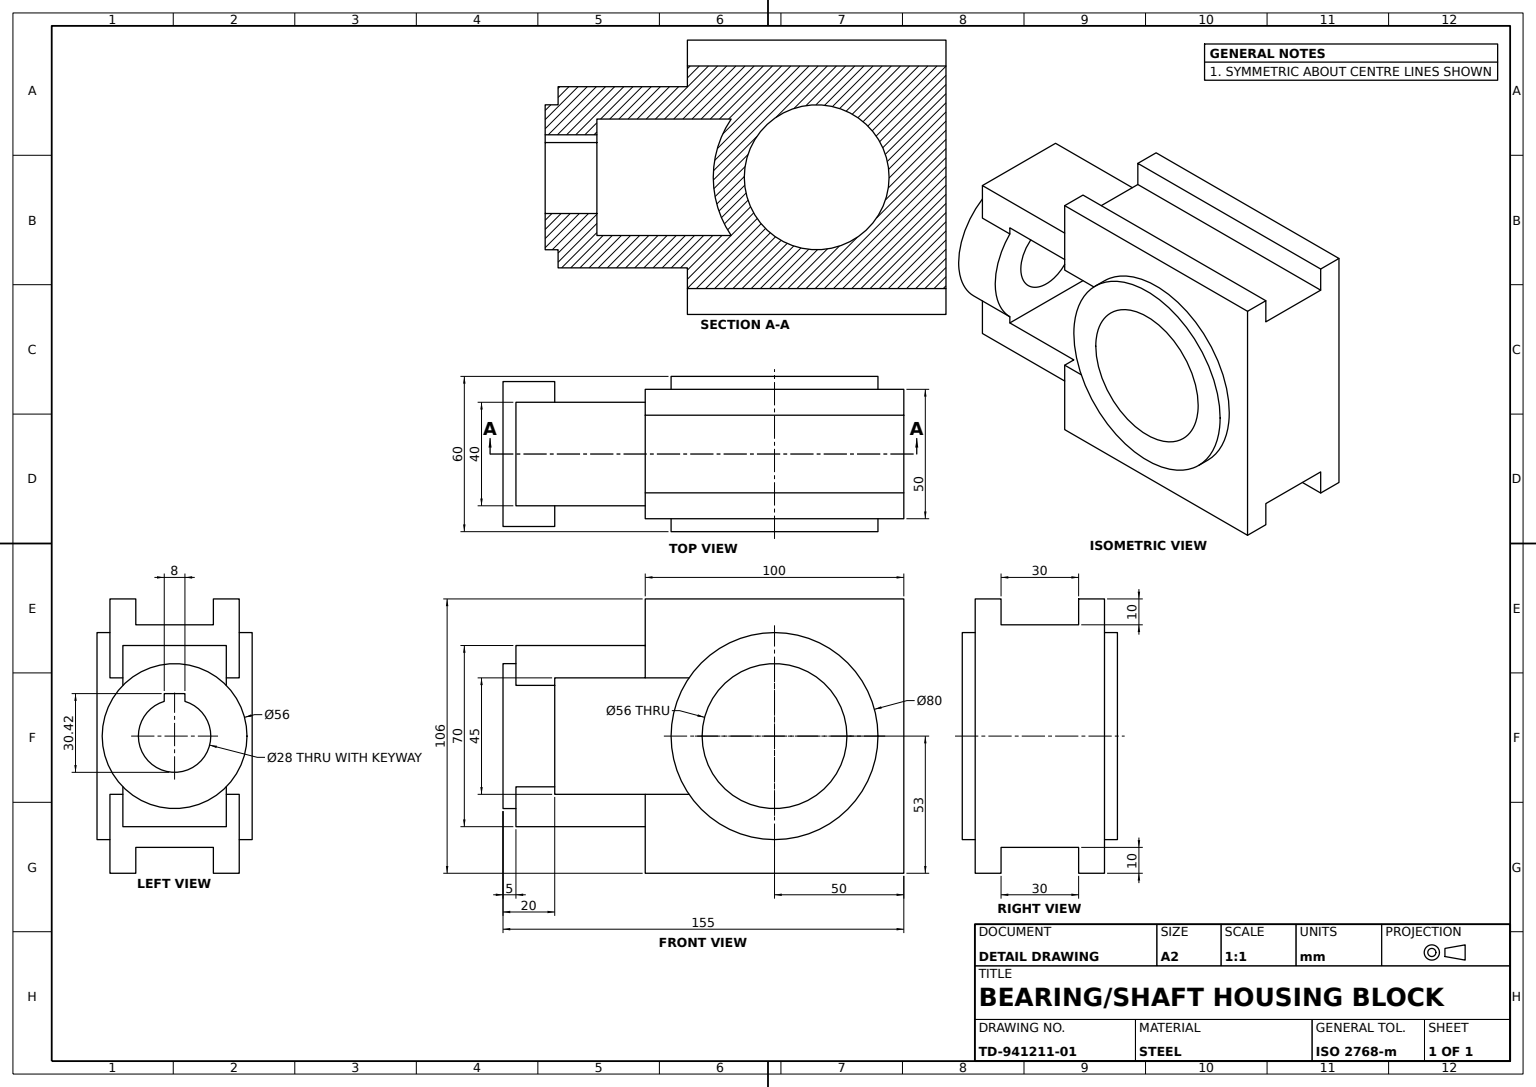
SolidWorks part; units mm, degrees
material "Plain Carbon Steel"
ref_plane "Front Plane" through (0, 0, 0) normal (0, 0, 1) x (1, 0, 0)
ref_plane "Top Plane" through (0, 0, 0) normal (0, 1, 0) x (1, 0, 0)
ref_plane "Right Plane" through (0, 0, 0) normal (1, 0, 0) x (0, 0, -1)
sketch "Base Block Profile" plane through (0, 0, 0) normal (0, 0, 1) x (1, 0, 0)
  line L1 (-50, -53) -> (50, -53)
  line L2 (-50, -53) -> (-50, 53)
  line L3 (-50, 53) -> (50, 53)
  line L4 (50, -53) -> (50, 53)
  line L5 (-50, -53) -> (50, 53) construction
  line L6 (-50, 53) -> (50, -53) construction
  point P0 (0, 0)
  dimension "D1" = 100
  dimension "D2" = 106
extrude "Base Block" add sketch "Base Block Profile" along normal mid plane 50
sketch "Housing Boss Profile" plane through (0, 0, 0) normal (0, 0, 1) x (1, 0, 0)
  line L0 (-50, 53) -> (-50, -53) construction
  line L1 (-50, 35) -> (-100, 35)
  line L2 (-50, 35) -> (-50, -35)
  line L3 (-50, -35) -> (-100, -35)
  line L4 (-100, 35) -> (-100, -35)
  point P7 (-100, 0)
  dimension "D1" = 100
  dimension "D2" = 70
extrude "Housing Boss" add sketch "Housing Boss Profile" along normal mid plane 40
sketch "Guide Key Slots Profile" plane through (-50, 0, 0) normal (-1, 0, 0) x (0, 0, 1)
  line L0 (25, 53) -> (-25, 53) construction
  line L1 (-15, 53) -> (15, 53)
  line L2 (-15, 53) -> (-15, 43)
  line L3 (-15, 43) -> (15, 43)
  line L4 (15, 53) -> (15, 43)
  line L5 (0, 0) -> (-49.9314, 0) construction
  line L6 (-15, -53) -> (-15, -43)
  line L7 (-15, -53) -> (15, -53)
  line L8 (-15, -43) -> (15, -43)
  line L9 (15, -53) -> (15, -43)
  point P6 (0, 43)
  dimension "D1" = 30
  dimension "D2" = 10
extrude "Guide Key Slots" cut sketch "Guide Key Slots Profile" against normal up to surface (100 mm away) up to face at (50, 0, 0)
sketch "Bearing Boss Profile Ø80" plane through (0, 0, 0) normal (0, 0, 1) x (1, 0, 0)
  circle A0 centre (0, 0) radius 40
  dimension "D1" = 80
extrude "Bearing Boss Ø80" add sketch "Bearing Boss Profile Ø80" along normal mid plane 60
sketch "Bearing Collar Profile Ø56" plane through (-100, 0, 0) normal (-1, 0, 0) x (0, 0, 1)
  circle A0 centre (0, 0) radius 28
  dimension "D1" = 56
extrude "Bearing Collar Ø56" add sketch "Bearing Collar Profile Ø56" against normal blind 15 and the other way blind 5
sketch "Bearing Bore Profile" plane through (0, 0, 0) normal (0, 0, 1) x (1, 0, 0)
  line L0 (-85, -19.5959) -> (-85, 19.5959) construction
  line L1 (-85, 22.5) -> (-33.0719, 22.5)
  line L2 (-85, 22.5) -> (-85, -22.5)
  line L3 (-85, -22.5) -> (-33.0719, -22.5)
  circle A0 centre (0, 0) radius 28
  circle A1 centre (0, 0) radius 40 construction
  circle A2 centre (0, 0) radius 40 construction
  arc A3 (-33.0719, 22.5) -> (-33.0719, -22.5) centre (0, 0) ccw
  point P12 (-85, 0)
  dimension "D1" = 56
  dimension "D2" = 45
extrude "Bearing Bore" cut sketch "Bearing Bore Profile" against normal through all both and the other way through all
sketch "Bore Keyway Profile" plane through (-105, 0, 0) normal (-1, 0, 0) x (0, 0, 1)
  line L2 (-4, 13.4164) -> (-4, 16.4164)
  line L3 (-4, 16.4164) -> (4, 16.4164)
  line L4 (4, 13.4164) -> (4, 16.4164)
  arc A0 (-4, 13.4164) -> (4, 13.4164) centre (0, 0) ccw
  point P1 (0, 16.4164)
  dimension "D3" = 14
  dimension "D1" = 8
  dimension "D2" = 3
extrude "Bore Keyway" cut sketch "Bore Keyway Profile" against normal up to surface (20 mm away) up to face at (-85, 0, 0)
